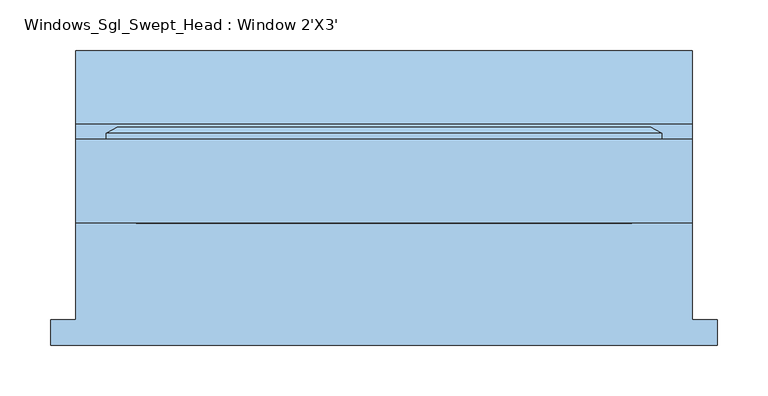
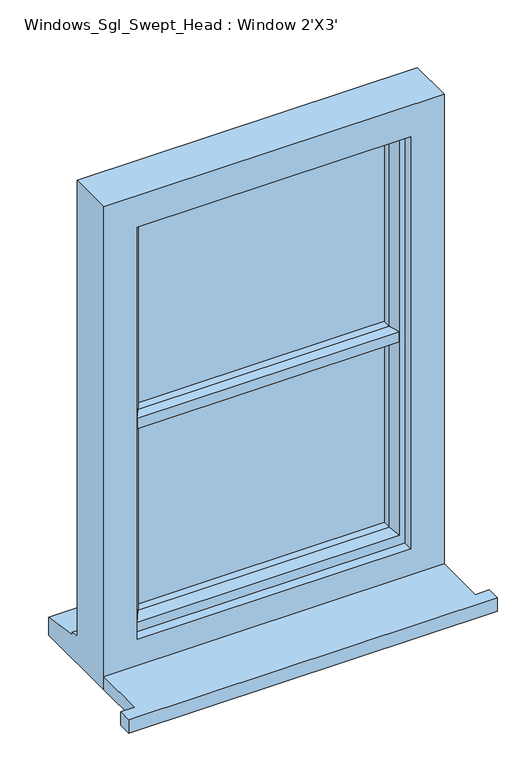
"""IFC4 building model written with IfcOpenShell, lengths in millimetres: window geometry, Windows_Sgl_Swept_Head : Window 2'X3'."""

from ifc_helpers import new_model, si_unit, point, frame, frame_2d, origin, place, context, project, spatial, polyline, circle_curve, trimmed, segment, composite_curve, outline, extrude, faceted_brep, source, transform, mapped, element, save


def windows_sgl_swept_head_window_2_x3_cc7253b0(model_context):
    return source(origin(), model_context, "Body", "SolidModel", [
        extrude(outline(polyline([(-329.8, -130.8434322), (-329.8, -105.8434322), (-304.8, -105.8434322), (-304.8, -10.2434322), (304.8, -10.2434322), (304.8, -105.8434322), (329.8, -105.8434322), (329.8, -130.8434322), (-329.8, -130.8434322)])), frame((0.0, 0.0, 1195.6), z_axis=(0.0, 0.0, 1.0), x_axis=(1.0, 0.0, 0.0)), (0.0, 0.0, 1.0), 25.0),
        faceted_brep([(-274.8, 72.7565678, 2080.0), (-274.8, 78.5300705, 2080.0), (-274.8, 78.5300705, 1248.6), (-274.8, 72.7565678, 1248.6), (-264.8, 7.7565678, 2070.0), (-264.8, 72.7565678, 2070.0), (-264.8, 72.7565678, 1258.6), (-264.8, 7.7565678, 1258.6), (-224.8, 22.2494677, 2030.0), (-234.9480377, 7.7565678, 2040.1480377), (-234.9480377, 7.7565678, 1288.4519623), (-224.8, 22.2494677, 1298.6), (-224.8, 36.7565678, 2030.0), (-224.8, 36.7565678, 1298.6), (-234.8, 60.7565678, 2040.0), (-234.8, 36.7565678, 2040.0), (-234.8, 36.7565678, 1288.6), (-234.8, 60.7565678, 1288.6), (-224.8, 78.5300705, 2030.0), (-224.8, 60.7565678, 2030.0), (-224.8, 60.7565678, 1298.6), (-224.8, 78.5300705, 1298.6), (-242.2457548, 84.3035732, 2047.4457548), (-242.2457548, 84.3035732, 1281.1542452), (-264.0153903, 84.3035732, 2069.2153903), (-264.0153903, 84.3035732, 1259.3846097), (274.8, 78.5300705, 1248.6), (274.8, 72.7565678, 1248.6), (264.8, 72.7565678, 1258.6), (264.8, 7.7565678, 1258.6), (234.9480377, 7.7565678, 1288.4519623), (224.8, 22.2494677, 1298.6), (224.8, 36.7565678, 1298.6), (234.8, 36.7565678, 1288.6), (234.8, 60.7565678, 1288.6), (224.8, 60.7565678, 1298.6), (224.8, 78.5300705, 1298.6), (242.2457548, 84.3035732, 1281.1542452), (264.0153903, 84.3035732, 1259.3846097), (274.8, 78.5300705, 2080.0), (274.8, 72.7565678, 2080.0), (264.8, 72.7565678, 2070.0), (264.8, 7.7565678, 2070.0), (234.9480377, 7.7565678, 2040.1480377), (224.8, 22.2494677, 2030.0), (224.8, 36.7565678, 2030.0), (234.8, 36.7565678, 2040.0), (234.8, 60.7565678, 2040.0), (224.8, 60.7565678, 2030.0), (224.8, 78.5300705, 2030.0), (242.2457548, 84.3035732, 2047.4457548), (264.0153903, 84.3035732, 2069.2153903)], [[[0, 1, 2, 3]], [[4, 5, 6, 7]], [[8, 9, 10, 11]], [[12, 8, 11, 13]], [[14, 15, 16, 17]], [[18, 19, 20, 21]], [[22, 18, 21, 23]], [[1, 24, 25, 2]], [[3, 2, 26, 27]], [[7, 6, 28, 29]], [[11, 10, 30, 31]], [[13, 11, 31, 32]], [[17, 16, 33, 34]], [[21, 20, 35, 36]], [[23, 21, 36, 37]], [[2, 25, 38, 26]], [[27, 26, 39, 40]], [[29, 28, 41, 42]], [[31, 30, 43, 44]], [[32, 31, 44, 45]], [[34, 33, 46, 47]], [[36, 35, 48, 49]], [[37, 36, 49, 50]], [[26, 38, 51, 39]], [[40, 39, 1, 0]], [[3, 27, 40, 0], [5, 41, 28, 6]], [[42, 41, 5, 4]], [[7, 29, 42, 4], [9, 43, 30, 10]], [[44, 43, 9, 8]], [[45, 44, 8, 12]], [[15, 46, 33, 16], [13, 32, 45, 12]], [[47, 46, 15, 14]], [[17, 34, 47, 14], [19, 48, 35, 20]], [[49, 48, 19, 18]], [[50, 49, 18, 22]], [[24, 51, 38, 25], [23, 37, 50, 22]], [[39, 51, 24, 1]]]),
        extrude(outline(polyline([(78.5300705, 1669.3), (78.5300705, 1659.3), (72.854277, 1649.3), (60.7565678, 1649.3), (60.7565678, 1656.3), (36.7565678, 1656.3), (36.7565678, 1649.3), (22.2494677, 1649.3), (7.7565678, 1654.4480377), (7.7565678, 1674.1519623), (22.2494677, 1679.3), (36.7565678, 1679.3), (36.7565678, 1672.3), (60.7565678, 1672.3), (60.7565678, 1679.3), (72.854277, 1679.3), (78.5300705, 1669.3)])), frame((-234.9480377, 0.0, 0.0), z_axis=(1.0, 0.0, 0.0), x_axis=(0.0, 1.0, 0.0)), (0.0, 0.0, 1.0), 469.8960754),
        extrude(outline(polyline([(234.9480377, 36.7565678), (-234.8, 36.7565678), (-234.8, 60.7565678), (234.9480377, 60.7565678), (234.9480377, 36.7565678)])), frame((0.0, 0.0, 1288.6), z_axis=(0.0, 0.0, 1.0), x_axis=(1.0, 0.0, 0.0)), (0.0, 0.0, 1.0), 370.5307627),
        extrude(outline(polyline([(234.9480377, 36.7565678), (-234.8, 36.7565678), (-234.8, 60.7565678), (234.9480377, 60.7565678), (234.9480377, 36.7565678)])), frame((0.0, 0.0, 1669.4692373), z_axis=(0.0, 0.0, 1.0), x_axis=(1.0, 0.0, 0.0)), (0.0, 0.0, 1.0), 370.5307627),
        faceted_brep([(-304.8, -10.2434322, 1195.6), (304.8, -10.2434322, 1195.6), (304.8, -10.2434322, 2110.0), (-304.8, -10.2434322, 2110.0), (-244.8, -10.2434322, 2050.0), (244.8, -10.2434322, 2050.0), (244.8, -10.2434322, 1270.6), (-244.8, -10.2434322, 1270.6), (-304.8, 72.7565678, 2110.0), (-304.8, 72.7565678, 1246.6), (-304.8, 87.7565678, 1245.28767), (-304.8, 87.7565678, 1240.3449676), (-304.8, 160.2565678, 1229.4088847), (-304.8, 160.2565678, 1195.6), (304.8, 72.7565678, 2110.0), (304.8, 72.7565678, 1246.6), (-264.8, 72.7565678, 2070.0), (-264.8, 72.7565678, 1258.6), (264.8, 72.7565678, 1258.6), (264.8, 72.7565678, 2070.0), (-264.8, 7.7565678, 2070.0), (-264.8, 7.7565678, 1258.6), (264.8, 7.7565678, 2070.0), (264.8, 7.7565678, 1258.6), (-244.8, 7.7565678, 2050.0), (-244.8, 7.7565678, 1270.6), (244.8, 7.7565678, 1270.6), (244.8, 7.7565678, 2050.0), (304.8, 160.2565678, 1195.6), (304.8, 160.2565678, 1229.4088847), (304.8, 87.7565678, 1240.3449676), (304.8, 87.7565678, 1245.28767)], [[[0, 1, 2, 3], [4, 5, 6, 7]], [[0, 3, 8, 9, 10, 11, 12, 13]], [[9, 8, 14, 15], [16, 17, 18, 19]], [[17, 16, 20, 21]], [[20, 22, 23, 21], [24, 25, 26, 27]], [[24, 4, 7, 25]], [[3, 2, 14, 8]], [[16, 19, 22, 20]], [[5, 4, 24, 27]], [[15, 14, 2, 1, 28, 29, 30, 31]], [[19, 18, 23, 22]], [[5, 27, 26, 6]], [[28, 1, 0, 13]], [[29, 28, 13, 12]], [[30, 29, 12, 11]], [[31, 30, 11, 10]], [[15, 31, 10, 9]], [[21, 23, 18, 17]], [[7, 6, 26, 25]]]),
        extrude(outline(composite_curve([segment(polyline([(1996.7836395, 224.8), (2030.0, 224.8), (2030.0, -224.8), (1996.7836395, -224.8)]), True, "CONTINUOUS"), segment(trimmed(circle_curve(frame_2d((1115.4, 0.0)), 909.6), [point((1996.7836395, -224.8))], [point((1996.7836395, 224.8))], True, "CARTESIAN"), True, "CONTINUOUS")], self_intersect=False)), frame((0.0, 48.7565678, 0.0), z_axis=(0.0, 1.0, 0.0), x_axis=(0.0, 0.0, 1.0)), (0.0, 0.0, 1.0), 24.0),
    ])


if __name__ == "__main__":
    model = new_model("IFC4")
    model_context = context("Model", 3, world=origin())
    ifc_project = project(units=[si_unit("LENGTHUNIT", "METRE", prefix="MILLI")], contexts=[model_context])
    site = spatial("IfcSite", under=ifc_project)
    building = spatial("IfcBuilding", under=site)
    placement = place(None, origin())
    windows_sgl_swept_head_window_2_x3_shape = windows_sgl_swept_head_window_2_x3_cc7253b0(model_context)
    element("IfcWindow", 1, ObjectType="Windows_Sgl_Swept_Head : Window 2'X3'", at=placement, inside=building, context=model_context, shape_type="MappedRepresentation", body=[
        mapped(windows_sgl_swept_head_window_2_x3_shape, transform((0.0, 0.0, 0.0), x_axis=(1.0, 0.0, 0.0), y_axis=(0.0, 1.0, 0.0), z_axis=(0.0, 0.0, 1.0))),
    ])
    save(model, "model.ifc")

# Revit data of these elements
# Type "Windows_Sgl_Swept_Head : Window 2'X3'"
#   Type Mark = "31"
#   Operation = "SinglePanel"
#   Construction Type Id = "SGL"
#   Manufacturer = "Revit"
#   Keynote = "L10"
#   Analytic Construction = "Large single-glazed windows"
#   Wrap Layers (Ext) from Ext = 0' - 4.03543"
#   Wrap Layers (Int) from Ext = 0' - 6.98819"
#   Window Board Projection = 0' - 0.98425"
#   Window Board Extension = 0' - 0.98425"
#   Visual Light Transmittance = 0.9
#   Solar Heat Gain Coefficient = 0.86
#   Rough Width = 2' - 0"
#   Rough Height = 3' - 0"
#   Radius - Swept Head = 2' - 11.81102"
#   Height = 3' - 0"
#   Width = 2' - 0"
#   Heat Transfer Coefficient (U) = 0.979472 BTU/(h·ft²·°F)
#   Glazing Thickness = 0' - 0.94488"
#   FrameOffset - External = 0' - 1.9685"
#   Frame Depth = 0' - 2.55906"
#   Default Head Height = 6' - 11.07087"
#   Cill Depth = 0' - 3.44488"
#   Cavity Closer Width = 0' - 1.9685"
#   Cavity Closer Offset from Ext = 0' - 4.03543"
#   Cavity Closer Depth = 0' - 3.34646"
#   Vis - Cavity Closers = yes
#   Define Thermal Properties by = 1
#   Material Trim = Window Frame
#   Material Glass = Glass
#   Material Frame = Window Frame
#   Wall Closure = (empty or 0)
# Element 1 (IfcWindow, "Windows_Sgl_Swept_Head : Window 2'X3'")
#   Materials on its faces: "Window Frame", "Glass"
# Materials
#   "Window Frame": colour RGB 249 249 249, transparency 0
#   "Glass": class "Glass", colour RGB 0 128 192, transparency 0.75, Description = "Soda Lime Glass", Cost = 0
